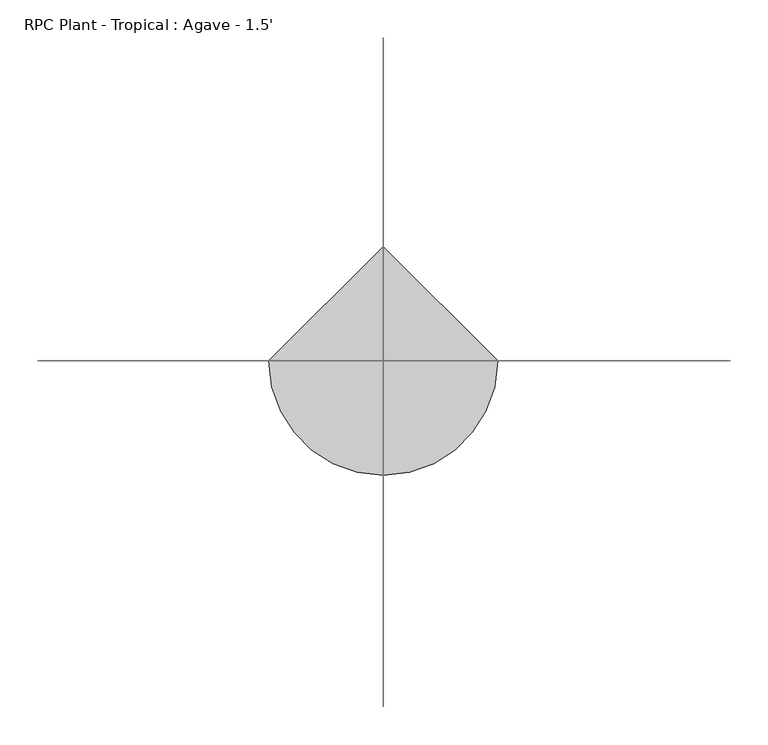
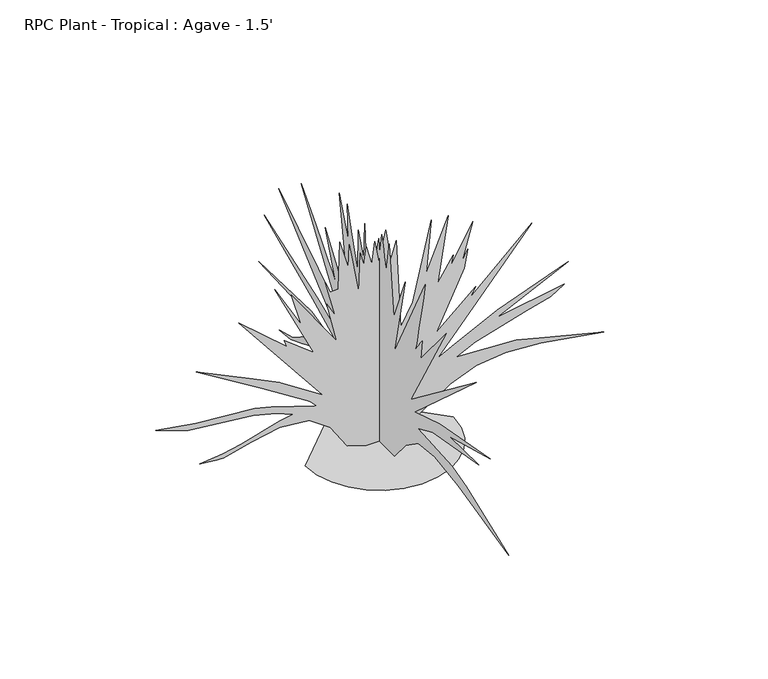
"""IFC4 building model written with IfcOpenShell, lengths in millimetres: geographic element geometry, RPC Plant - Tropical : Agave - 1.5'."""

from ifc_helpers import new_model, si_unit, origin, place, context, project, spatial, triangles, source, transform, mapped, element, save


def rpc_plant_tropical_agave_1_5_93a2a214(model_context):
    return source(origin(), model_context, "Body", "Tessellation", [
        triangles([(-150.7087333, 0.0, 9.4e-06), (-146.7244834, -34.5323444, 9.4e-06), (-135.3772836, -66.2450299, 9.4e-06), (-117.5759356, -94.2289958, 9.4e-06), (-94.2289958, -117.5759356, 9.4e-06), (-66.2450299, -135.3772836, 9.4e-06), (-34.5323444, -146.7244834, 9.4e-06), (6.6e-06, -150.7087333, 9.4e-06), (34.5323444, -146.7244834, 9.4e-06), (66.2450299, -135.3772836, 9.4e-06), (94.2289958, -117.5759356, 9.4e-06), (117.5759356, -94.2289958, 9.4e-06), (135.3772836, -66.2450299, 9.4e-06), (146.7244834, -34.5323444, 9.4e-06), (150.7087333, 1.32e-05, 9.4e-06), (-1.98e-05, 150.7087333, 9.4e-06), (-24.9398476, 1.1e-06, 2.5e-06), (-65.4258802, 2.1e-06, 13.141818), (-99.6620581, 5e-07, 65.0964399), (-143.0435126, 6e-07, 95.6658721), (-202.3246234, 2.8e-06, 101.1403381), (-259.7355268, 6e-06, 89.1792132), (-316.7763402, 9.4e-06, 74.9889865), (-329.6211594, 9.9e-06, 75.5035945), (-365.3285002, 1.12e-05, 79.1975187), (-318.313056, 8.9e-06, 84.1103911), (-282.3389982, 6.9e-06, 91.7898278), (-203.1008479, 2e-06, 114.8573697), (-175.7107319, 5e-07, 119.829677), (-208.3624635, 1.2e-06, 133.0887423), (-256.7688111, 2.5e-06, 145.787731), (-389.2832517, 7.5e-06, 160.0767662), (-455.2115313, 9e-06, 182.6248811), (-373.9467241, 6.3e-06, 169.0808314), (-253.2813787, 1.6e-06, 159.2306877), (-220.3573709, 6e-07, 151.0805947), (-127.6907252, -1.6e-06, 121.0610699), (-140.4735387, -1.9e-06, 135.3043865), (-238.3492232, -1.3e-06, 197.06021), (-372.7148226, -4e-07, 279.8955245), (-256.342093, -2.1e-06, 224.048243), (-204.0302424, -2.9e-06, 198.6317166), (-115.3780683, -3.3e-06, 140.7615752), (-286.5249345, -8.6e-06, 355.0033673), (-188.0233888, -7.9e-06, 270.045399), (-192.9487059, -8.5e-06, 284.8205873), (-133.8471808, -8.3e-06, 238.0324729), (-212.6492294, -1.47e-05, 401.7927715), (-158.472758, -1.14e-05, 306.9846414), (-179.4046562, -1.47e-05, 378.3993593), (-87.0585669, -1.09e-05, 246.6514781), (-106.7590813, -1.52e-05, 332.8418567), (-89.5210982, -1.41e-05, 302.0595786), (-110.4530055, -1.79e-05, 380.860619), (-99.717687, -1.69e-05, 356.9287222), (-83.2732056, -1.76e-05, 356.9490335), (-80.9021112, -2.37e-05, 457.2003633), (-63.426897, -2.09e-05, 396.9718449), (-61.2016014, -2.38e-05, 444.8864347), (-41.5013458, -1.82e-05, 335.3031163), (-39.0385601, -2.33e-05, 419.0317629), (-31.650966, -2.19e-05, 390.7107445), (-26.7259009, -2.44e-05, 428.8818884), (-15.6443803, -2.24e-05, 387.0175833), (-9.4879996, -2.54e-05, 433.8069511), (-0.8690236, -2.3e-05, 387.0175833), (12.6750416, -2.74e-05, 451.043399), (23.7565623, -2.39e-05, 383.3244221), (34.8381601, -2.66e-05, 420.261121), (43.4571494, -1.56e-05, 230.6448788), (68.0824677, -1.94e-05, 276.2023633), (105.4982208, -3.08e-05, 439.9537416), (95.1708261, -2.38e-05, 329.146152), (140.4829403, -3.22e-05, 436.9539974), (118.5650104, -2.3e-05, 299.5957755), (150.578436, -2.74e-05, 348.8489465), (145.6533642, -2.58e-05, 326.6848924), (189.9794467, -3.25e-05, 406.7178343), (167.81641, -2.69e-05, 327.9167939), (180.1290669, -2.88e-05, 351.3102061), (173.4681726, -2.62e-05, 313.009528), (116.102479, -1.66e-05, 193.7063995), (196.1359024, -2.44e-05, 265.1203362), (183.8229911, -2.26e-05, 244.1889286), (310.6447741, -3.51e-05, 361.1603316), (118.5650104, -1.34e-05, 138.2987895), (158.4747927, -1.63e-05, 158.0775423), (240.4617396, -2.24e-05, 198.6317166), (384.5207517, -3.19e-05, 252.8079337), (239.2306011, -2.13e-05, 182.6248811), (376.7864491, -2.88e-05, 206.3655105), (349.174072, -2.66e-05, 189.8819236), (300.4111145, -2.36e-05, 176.0696308), (195.4584909, -1.73e-05, 146.0828801), (156.7348917, -1.44e-05, 127.2172711), (278.6305944, -1.94e-05, 121.0610699), (336.3953462, -2.1e-05, 106.1004551), (457.1673348, -2.45e-05, 75.5035945), (329.0750444, -2.01e-05, 96.2046111), (257.431743, -1.73e-05, 101.1027496), (197.4574787, -1.42e-05, 94.105802), (144.7537007, -1.07e-05, 73.3684686), (86.5066293, -5.8e-06, 34.1325482), (33.0588878, -1.4e-06, 0.0), (9e-07, 20.0836192, 9.1e-06), (2.1e-06, 47.8000438, 9.9e-06), (3.7e-06, 68.4088604, 20.0829062), (6.2e-06, 99.6950775, 59.1195655), (8.3e-06, 132.7178983, 80.7177112), (1.03e-05, 174.2748821, 84.8467378), (1.15e-05, 208.5839434, 72.8693576), (1.35e-05, 272.2425033, 45.8366235), (1.48e-05, 311.9833551, 30.2844433), (1.65e-05, 353.3269798, 25.0212039), (1.48e-05, 305.3793614, 38.860505), (1.34e-05, 249.7515432, 74.8251566), (1.18e-05, 199.8564965, 97.660536), (1.01e-05, 161.2479701, 96.4354927), (1.17e-05, 188.527337, 110.366392), (1.51e-05, 256.1160167, 122.0234748), (2.29e-05, 425.717038, 129.5510222), (1.47e-05, 238.8183625, 134.6051196), (1.09e-05, 164.9452008, 118.743824), (8.2e-06, 119.3844099, 96.4354927), (1.1e-05, 159.9457058, 127.6671074), (1.54e-05, 233.8196305, 165.2718342), (2.53e-05, 406.273312, 240.4952587), (1.5e-05, 217.8867004, 177.6998184), (1.1e-05, 147.7036569, 148.1491784), (2.57e-05, 354.5588814, 329.146152), (1.25e-05, 146.2032761, 198.5547591), (2.38e-05, 274.5259576, 388.2494848), (2.18e-05, 248.7817623, 359.4966614), (1.99e-05, 223.9913424, 331.6328098), (1.81e-05, 201.1074557, 305.5495545), (1.65e-05, 181.0833509, 282.1358129), (1.52e-05, 164.872549, 262.2780679), (1.42e-05, 153.4283166, 246.8711776), (1.37e-05, 147.7036569, 236.8013344), (1.88e-05, 190.798601, 345.1532418), (1.51e-05, 148.9134577, 283.7461616), (1.48e-05, 144.9251474, 278.3410409), (1.44e-05, 140.1001603, 272.7403471), (1.4e-05, 134.5776867, 266.9770725), (1.35e-05, 128.4971803, 261.086807), (1.31e-05, 121.9980766, 255.0974924), (1.26e-05, 115.2200837, 249.0439011), (1.21e-05, 108.3028915, 242.95779), (1.97e-05, 140.3160628, 449.8114975), (1.58e-05, 109.53403, 367.3172959), (1.82e-05, 113.2279542, 442.4251751), (1.61e-05, 98.452766, 393.1745476), (1.29e-05, 75.0583319, 320.5279281), (1.55e-05, 73.826939, 410.4109955), (1.32e-05, 55.357822, 358.699072), (1.53e-05, 51.6638932, 437.5001123), (1.36e-05, 47.2595336, 384.1829453), (1.1e-05, 27.0383205, 327.9167939), (1.31e-05, 1.1814591, 436.2682108), (1.2e-05, -1.2811313, 405.4859327), (1.3e-05, -8.5500533, 450.4566616), (1.25e-05, -11.9783704, 436.1437634), (1.19e-05, -15.2441015, 422.2677209), (1.14e-05, -18.1847128, 409.2629188), (1.09e-05, -20.6375916, 397.5687561), (1.05e-05, -22.4401819, 387.6195451), (1.03e-05, -23.4298925, 379.852214), (1.01e-05, -23.4441676, 374.7036547), (1.18e-05, -34.5257405, 446.1183363), (6.6e-06, -50.5323262, 298.3664174), (7.8e-06, -92.3958773, 399.3315119), (4.4e-06, -52.9948575, 225.7198161), (5.7e-06, -162.5786665, 436.2682108), (5.1e-06, -155.9520543, 404.0000133), (4.4e-06, -149.5159464, 372.9078704), (3.8e-06, -143.4613468, 344.1651844), (3.3e-06, -137.9787509, 318.9480463), (2.9e-06, -133.2591716, 298.4324563), (2.7e-06, -129.4933677, 283.7918891), (2.6e-06, -126.87158, 276.2023633), (2.5e-06, -126.0089964, 274.2135312), (2.5e-06, -127.1682462, 275.2524031), (2.5e-06, -130.0120315, 278.8160301), (2.5e-06, -134.204054, 284.398956), (2.5e-06, -139.4067433, 291.4957067), (2.4e-06, -145.2835467, 299.6034059), (2.4e-06, -151.4971481, 308.2165429), (1.4e-06, -145.3409469, 266.3522378), (6e-07, -236.4556433, 375.9355562), (-2e-07, -110.8649898, 157.9992949), (-5.3e-06, -341.1146439, 334.0712148), (-1.4e-06, -124.4090487, 138.2990438), (-4.6e-06, -213.0612137, 166.6183), (-1.15e-05, -391.2898516, 199.4396978), (-6.2e-06, -246.3057688, 160.4618262), (-1.09e-05, -351.4651749, 162.9246119), (-4.5e-06, -189.3266705, 133.5012353), (-2.8e-06, -135.490567, 109.9795515), (-8.4e-06, -257.3885589, 102.5916939), (-1.11e-05, -306.6392046, 89.0476442), (-1.94e-05, -455.623025, 31.1775097), (-1.03e-05, -278.0057598, 72.8693576), (-6.2e-06, -195.1343828, 85.0082832), (-3.8e-06, -137.6096873, 78.9734862), (-2.8e-06, -94.1832773, 48.8668437), (-2.4e-06, -52.6021717, 6.9e-06), (-9e-07, -19.1255291, 7.9e-06)], [[15, 16, 1], [14, 15, 1], [14, 1, 2], [13, 14, 2], [13, 2, 3], [13, 3, 4], [12, 13, 4], [11, 12, 4], [11, 4, 5], [11, 5, 6], [11, 6, 7], [11, 7, 8], [11, 8, 9], [11, 9, 10], [47, 48, 49], [97, 98, 99], [88, 89, 90], [39, 40, 41], [84, 85, 86], [71, 72, 73], [53, 54, 55], [32, 33, 34], [43, 44, 45], [24, 25, 26], [58, 59, 60], [77, 78, 79], [73, 74, 75], [60, 61, 62], [51, 52, 53], [56, 57, 58], [82, 83, 84], [79, 80, 81], [64, 65, 66], [49, 50, 51], [68, 69, 70], [75, 76, 77], [90, 91, 92], [90, 92, 93], [66, 67, 68], [82, 84, 86], [90, 93, 94], [62, 63, 64], [47, 49, 51], [39, 41, 42], [45, 46, 47], [43, 45, 47], [38, 39, 42], [38, 42, 43], [31, 32, 34], [31, 34, 35], [23, 24, 26], [56, 58, 60], [87, 88, 90], [87, 90, 94], [87, 94, 95], [37, 38, 43], [86, 87, 95], [71, 73, 75], [96, 97, 99], [96, 99, 100], [95, 96, 100], [95, 100, 101], [95, 101, 102], [53, 55, 56], [53, 56, 60], [22, 23, 26], [22, 26, 27], [22, 27, 28], [21, 22, 28], [60, 62, 64], [43, 47, 51], [30, 31, 35], [30, 35, 36], [30, 36, 37], [29, 30, 37], [86, 95, 102], [21, 28, 29], [20, 21, 29], [20, 29, 37], [19, 20, 37], [86, 102, 103], [66, 68, 70], [64, 66, 70], [60, 64, 70], [53, 60, 70], [51, 53, 70], [43, 51, 70], [77, 79, 81], [77, 81, 82], [75, 77, 82], [71, 75, 82], [70, 71, 82], [70, 82, 86], [43, 70, 86], [43, 86, 103], [43, 103, 104], [43, 104, 17], [43, 17, 18], [43, 18, 19], [43, 19, 37], [120, 121, 122], [193, 194, 195], [190, 191, 192], [126, 127, 128], [155, 156, 157], [131, 132, 133], [200, 201, 202], [113, 114, 115], [195, 196, 197], [129, 130, 131], [131, 133, 134], [170, 171, 172], [188, 189, 190], [131, 134, 135], [148, 149, 150], [139, 140, 141], [131, 135, 136], [150, 151, 152], [168, 169, 170], [172, 173, 174], [131, 136, 137], [158, 159, 160], [172, 174, 175], [131, 137, 138], [153, 154, 155], [131, 138, 139], [172, 175, 176], [160, 161, 162], [172, 176, 177], [186, 187, 188], [172, 177, 178], [112, 113, 115], [112, 115, 116], [111, 112, 116], [111, 116, 117], [160, 162, 163], [172, 178, 179], [172, 179, 180], [172, 180, 181], [139, 141, 142], [193, 195, 197], [185, 186, 188], [192, 193, 197], [192, 197, 198], [155, 157, 158], [150, 152, 153], [148, 150, 153], [139, 142, 143], [199, 200, 202], [119, 120, 122], [119, 122, 123], [118, 119, 123], [199, 202, 203], [198, 199, 203], [198, 203, 204], [184, 185, 188], [110, 111, 117], [110, 117, 118], [109, 110, 118], [160, 163, 164], [118, 123, 124], [109, 118, 124], [139, 143, 144], [125, 126, 128], [125, 128, 129], [183, 184, 188], [139, 144, 145], [153, 155, 158], [108, 109, 124], [139, 145, 146], [160, 164, 165], [158, 160, 165], [158, 165, 166], [158, 166, 167], [158, 167, 168], [158, 168, 170], [182, 183, 188], [124, 125, 129], [182, 188, 190], [181, 182, 190], [172, 181, 190], [139, 146, 147], [131, 139, 147], [131, 147, 148], [158, 170, 172], [153, 158, 172], [148, 153, 172], [198, 204, 205], [131, 148, 172], [129, 131, 172], [124, 129, 172], [124, 172, 190], [108, 124, 190], [107, 108, 190], [106, 107, 190], [105, 106, 190], [207, 105, 190], [206, 207, 190], [205, 206, 190], [198, 205, 190], [192, 198, 190]], closed=False),
    ])


if __name__ == "__main__":
    model = new_model("IFC4")
    model_context = context("Model", 3, world=origin())
    ifc_project = project(units=[si_unit("LENGTHUNIT", "METRE", prefix="MILLI")], contexts=[model_context])
    site = spatial("IfcSite", under=ifc_project)
    building = spatial("IfcBuilding", under=site)
    placement = place(None, origin())
    rpc_plant_tropical_agave_1_5_shape = rpc_plant_tropical_agave_1_5_93a2a214(model_context)
    element("IfcGeographicElement", 1, ObjectType="RPC Plant - Tropical : Agave - 1.5'", at=placement, inside=building, context=model_context, shape_type="MappedRepresentation", body=[
        mapped(rpc_plant_tropical_agave_1_5_shape, transform((0.0, 0.0, 0.0), x_axis=(1.0, 0.0, 0.0), y_axis=(0.0, 1.0, 0.0), z_axis=(0.0, 0.0, 1.0))),
    ])
    save(model, "model.ifc")

# Revit data of these elements
# Type "RPC Plant - Tropical : Agave - 1.5'"
#   built-in parameter 1005198 = "{2, 15},{39, RPC-16-G1GJ-63FX-7K5P-N000-ST1L-LVER-AU},{1, 0},{1, 0},{2, 13},{1, 8},{5, Color},{1, 0},{1, 0},{3, 0.8},{3, 0.8},{3, 0.8},{1, 8},{7, BBoxMin},{1, 0},{1, 0},{1, 0},{1, 0},{1, 0},{1, 8},{7, BBoxMax},{1, 0},{1, 0},{1, 0},{1, 0},{1, 0},{2, 11},{9, RPCTypeId},{1, 0},{1, 0},{39, RPC-16-G1GJ-63FX-7K5P-N000-ST1L-LVER-AU},{1, 6},{14, RPCPlantHeight},{1, 0},{1, 0},{3, 1.5},{2, 11},{7, keyword},{1, 0},{1, 0},{35, :RPCs:Plants [General]:Geometry:RPC},{2, 11},{8, category},{1, 0},{1, 0},{16, Plants [General]},{2, 11},{12, LocalizedUID},{1, 0},{1, 0},{5, Agave},{2, 14},{6, Height},{1, 0},{1, 0},{3, 1.5},{1, 2},{16, Cast Reflections},{1, 0},{1, 0},{1, 0},{1, 2},{12, Cast Shadows},{1, 0},{1, 0},{1, 1},{1, 2},{9, Lock View},{1, 0},{1, 0},{1, 0},{1, 4},{5, ViewC},{1, 0},{1, 0},{1, 0},{21, assetlibrary_base.fbx},{1, 5},"
#   built-in parameter 1005195 = "RPC-16-G1GJ-63FX-7K5P-N000-ST1L-LVER-AU"
#   Type Comments = "Agave"
#   Assembly Code = "G2050500"
#   Height = 1' - 6"
#   Default Elevation = 0
